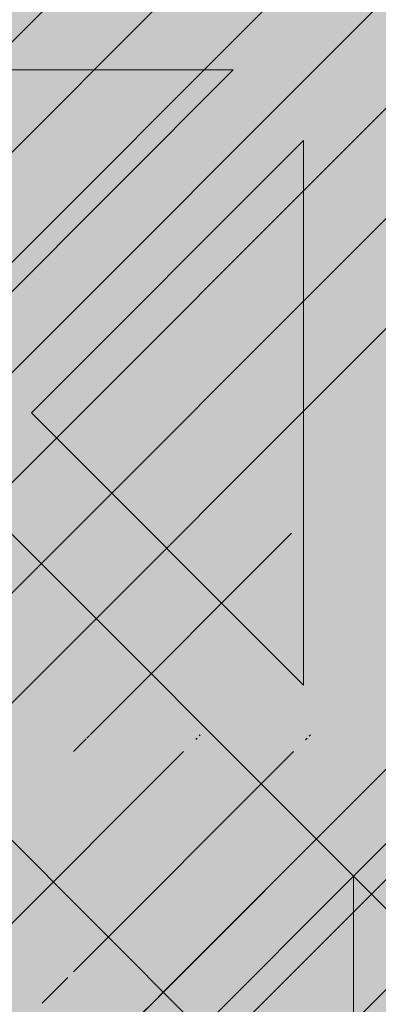
# Model space of a CAD drawing. Units: inches. Extents: x 844 to 2234, y 346 to 1084.
# Tile 11 of 93: x 1122.002 to 1122.921, y 691.183 to 693.702. Entities that reach past the tile are written whole.
import ezdxf

# ---------------------------------------------------------------- set-up
doc = ezdxf.new("R2010")
doc.units = ezdxf.units.IN
doc.header["$MEASUREMENT"] = 0
for name, color, linetype, lineweight in [('A-ANNO-DIMS', 2, 'Continuous', 18), ('furniture', 8, 'Continuous', 18), ('RA-AP-01$0$INT', 35, 'Continuous', 5)]:
    doc.layers.add(name, color=color, linetype=linetype, lineweight=lineweight)
doc.layers.add('RA-AP-01$0$FURN', color=3, linetype='Continuous')
doc.layers.add('RA-AP-01$0$WOOD', color=64, linetype='Continuous')
doc.styles.get("Standard").update_dxf_attribs({"font": 'arial.ttf'})
doc.dimstyles.get("Standard").update_dxf_attribs({"dimtxt": 6, "dimasz": 3, "dimexe": 0.18, "dimexo": 0.0625, "dimgap": 0.09, "dimtad": 0, "dimtih": 1, "dimtoh": 1, "dimdec": 1, "dimzin": 0, "dimdsep": 46, "dimlunit": 3, "dimtxsty": 'Standard', "dimblk": 'ARCHTICK', "dimcen": 0.09, "dimadec": 0, "dimazin": 0, "dimtfac": 1, "dimtdec": 1, "dimtofl": 0, "dimtmove": 0, "dimatfit": 3, "dimfxl": 1, "dimtolj": 1, "dimtzin": 0, "dimarcsym": 0})

# ---------------------------------------------------------------- blocks, each defined once
blk = doc.blocks.new('A$C18D01794')
at = {"layer": 'RA-AP-01$0$INT'}
h = blk.add_hatch(color=256, dxfattribs=at)
h.paths.add_polyline_path([(4.585917135068449, -6.356712009588271), (4.555206456959269, -6.35671200958746), (4.555206456959137, -6.387422687716308), (4.874495778835233, -6.706712009592356), (4.90520645695423, -6.676001331474049)])
h.paths.add_polyline_path([(5.255206456948813, -6.387422687716306), (5.255206456948682, -6.356712009605972), (5.224495778822613, -6.356712009605161), (4.905206456953498, -6.676001331474273), (4.935917135072151, -6.706712009592924)])
h.paths.add_polyline_path([(4.935917135072559, -6.706712009592068), (4.905206456953564, -6.737422687710376), (5.255206456951813, -7.087422687708613), (5.255206456951549, -7.026001331471008)])
h.paths.add_polyline_path([(4.555206456956399, -7.026001331471013), (4.555206456956134, -7.087422687708616), (4.905206456953821, -6.737422687710943), (4.874495778835166, -6.70671200959229)])
h = blk.add_hatch(color=256, dxfattribs=at)
h.paths.add_polyline_path([(4.585917135068448, -6.356712009588273), (4.614201406330596, -6.356712009589021), (4.668846067270487, -6.411356670531338), (4.723490728212344, -6.356712009591912), (4.771774999457151, -6.35671200959319), (4.826419660396886, -6.411356670535356), (4.862780050090322, -6.374996280843536), (4.844495778842715, -6.356712009595112), (4.862780050090411, -6.356712009595595), (4.905206456960182, -6.399138416468211), (4.947632863832445, -6.356712009597838), (4.965917135079675, -6.356712009598322), (4.947632863831759, -6.374996280845421), (4.983993253523576, -6.411356670538857), (5.038637914464627, -6.356712009600247), (5.08692218571208, -6.356712009601523), (5.141566846649976, -6.411356670541852), (5.196211507589851, -6.356712009604411), (5.224495778822615, -6.356712009605161), (4.905206456953975, -6.676001331473793)])
h.paths.add_polyline_path([(4.895206456956031, -6.637717060225675), (4.895206456958921, -6.528427738347902), (4.840561796018589, -6.583072399285802)], flags=16)
h.paths.add_polyline_path([(4.915206456955638, -6.637717060226121), (4.969851117895509, -6.583072399288678), (4.915206456957609, -6.528427738348344)], flags=16)
h.paths.add_polyline_path([(4.826419660395175, -6.568930263661755), (4.881064321335613, -6.514285602723745), (4.771774999456703, -6.514285602720857)], flags=16)
h.paths.add_polyline_path([(4.983993253519558, -6.568930263665262), (5.038637914460456, -6.514285602726792), (4.929348592581548, -6.514285602724816)], flags=16)
h.paths.add_polyline_path([(4.881064321336025, -6.494285602723742), (4.826419660397532, -6.439640941782821), (4.771774999457062, -6.494285602720859)], flags=16)
h.paths.add_polyline_path([(4.929348592582019, -6.494285602724817), (5.038637914460982, -6.494285602726792), (4.983993253522945, -6.439640941786327)], flags=16)
h.paths.add_polyline_path([(4.895206456960191, -6.480143467100443), (4.895206456962115, -6.407422687715913), (4.876922185715016, -6.389138416467584), (4.840561796021581, -6.425498806159401)], flags=16)
h.paths.add_polyline_path([(4.915206456958487, -6.480143467100889), (4.969851117899527, -6.425498806162279), (4.933490728206909, -6.389138416468043), (4.9152064569598, -6.40742268771434)], flags=16)
h.paths.add_polyline_path([(4.757632863832376, -6.480143467096812), (4.812277524772842, -6.425498806158772), (4.757632863834348, -6.370854145217844)], flags=16)
h.paths.add_polyline_path([(4.737632863832376, -6.480143467096286), (4.737632863834348, -6.370854145217375), (4.682988202893906, -6.425498806155385)], flags=16)
h.paths.add_polyline_path([(5.05278005008503, -6.480143467103376), (5.052780050087917, -6.370854145224413), (4.998135389146995, -6.425498806162908)], flags=16)
h.paths.add_polyline_path([(5.072780050085024, -6.480143467103744), (5.127424711025931, -6.42549880616527), (5.072780050087916, -6.370854145224832)], flags=16)
h.paths.add_polyline_path([(4.935917135072783, -6.706712009592292), (5.255206456948811, -6.387422687716309), (5.255206456948932, -6.415706958964177), (5.200561796010279, -6.470351619902839), (5.255206456949403, -6.524996280841948), (5.25520645694961, -6.5732805520894), (5.200561796009787, -6.627925213029239), (5.236922185702417, -6.664285602721864), (5.255206456949919, -6.646001331474357), (5.255206456949998, -6.664285602721898), (5.212780050078687, -6.706712009592262), (5.25520645695036, -6.749138416463932), (5.255206456950438, -6.767422687711313), (5.236922185702424, -6.749138416463297), (5.200561796009796, -6.785498806155928), (5.255206456950753, -6.840143467096874), (5.25520645695096, -6.888427738341682), (5.200561796010322, -6.943072399282328), (5.255206456951428, -6.997717060223427), (5.255206456951547, -7.026001331471006)])
h.paths.add_polyline_path([(5.042988202883395, -6.785498806155427), (5.097632863823085, -6.840143467095101), (5.097632863822622, -6.730854145216193)], flags=16)
h.paths.add_polyline_path([(5.028846067259663, -6.771356670531693), (5.083490728198774, -6.716712009592573), (4.974201406321001, -6.716712009593042)], flags=16)
h.paths.add_polyline_path([(5.117632863823087, -6.840143467095186), (5.172277524762331, -6.785498806155926), (5.11763286382262, -6.730854145216225)], flags=16)
h.paths.add_polyline_path([(5.08349072819877, -6.696712009593886), (5.028846067259652, -6.642067348654775), (4.974201406320998, -6.696712009593438)], flags=16)
h.paths.add_polyline_path([(5.131774999446817, -6.854285602718917), (5.186419660386065, -6.799640941779662), (5.241064321325782, -6.854285602719365)], flags=17)
h.paths.add_polyline_path([(5.131774999446228, -6.716712009592374), (5.186419660386065, -6.771356670532194), (5.222780050079488, -6.734996280838764), (5.204495778832781, -6.716712009592063)], flags=16)
h.paths.add_polyline_path([(5.097632863822613, -6.682569873970264), (5.097632863823061, -6.573280552091354), (5.042988202883383, -6.627925213031044)], flags=16)
h.paths.add_polyline_path([(5.131774999446899, -6.874285602718915), (5.241064321325809, -6.874285602719364), (5.186419660386591, -6.928930263658598)], flags=17)
h.paths.add_polyline_path([(5.131774999446226, -6.696712009594078), (5.204495778830767, -6.696712009594374), (5.22278005007868, -6.67842773834687), (5.186419660386049, -6.642067348654249)], flags=16)
h.paths.add_polyline_path([(5.11763286382262, -6.682569873970225), (5.17227752476232, -6.627925213030515), (5.117632863823064, -6.573280552091267)], flags=16)
h.paths.add_polyline_path([(5.186419660386069, -6.613783077405491), (5.241064321325754, -6.559138416465795), (5.131774999446791, -6.559138416466263)], flags=16)
h.paths.add_polyline_path([(5.131774999446872, -6.539138416466263), (5.24106432132578, -6.539138416465794), (5.186419660386554, -6.484493755526573)], flags=16)
h.paths.add_polyline_path([(5.255206456951811, -7.08742268770861), (5.255206456951895, -7.106712009588038), (4.555206456956052, -7.106712009588038), (4.555206456956136, -7.087422687708617), (4.905206456953973, -6.737422687710788)])
h.paths.add_polyline_path([(4.983993253513404, -6.8444937555241), (4.92934859257295, -6.899138416462108), (5.03863791445186, -6.899138416465014)], flags=16)
h.paths.add_polyline_path([(4.969851117889988, -6.83035161990006), (4.915206456952556, -6.775706958960171), (4.915206456949648, -6.884996280837944)], flags=16)
h.paths.add_polyline_path([(4.929348592572535, -6.919138416462105), (4.983993253511019, -6.973783077403037), (5.038637914451496, -6.919138416465012)], flags=16)
h.paths.add_polyline_path([(5.052780050074912, -6.93328055208906), (4.998135389134438, -6.987925213027088), (5.052780050072919, -7.042569873968025)], flags=16)
h.paths.add_polyline_path([(5.07278005007491, -6.933280552089588), (5.072780050072918, -7.042569873968497), (5.127424711013374, -6.987925213030498)], flags=16)
h.paths.add_polyline_path([(4.89520645695295, -6.775706958959721), (4.840561796013067, -6.830351619897157), (4.895206456950961, -6.884996280837494)], flags=16)
h.paths.add_polyline_path([(4.915206456948365, -6.933280552085403), (4.915206456946434, -7.006001331471951), (4.933490728192729, -7.024285602719066), (4.969851117886972, -6.987925213026453)], flags=16)
h.paths.add_polyline_path([(4.881064321327021, -6.899138416461022), (4.82641966038902, -6.84449375552057), (4.771774999448108, -6.899138416459029)], flags=16)
h.paths.add_polyline_path([(4.895206456950073, -6.933280552084951), (4.840561796009022, -6.987925213023558), (4.876922185700835, -7.024285602716997), (4.895206456948749, -7.006001331469487)], flags=16)
h.paths.add_polyline_path([(4.983993253510392, -7.0020673486505), (4.947632863816944, -7.038427738342319), (4.965917135064043, -7.05671200959023), (5.038637914448995, -7.056712009591555)], flags=16)
h.paths.add_polyline_path([(4.881064321326543, -6.91913841646102), (4.771774999447578, -6.919138416459031), (4.826419660385607, -6.973783077399508)], flags=16)
h.paths.add_polyline_path([(4.905206456946447, -7.014285602717636), (4.862780050074785, -7.056712009588352), (4.947632863816685, -7.056712009589775)], flags=16)
h.paths.add_polyline_path([(5.14156684663679, -7.002067348654549), (5.086922185696452, -7.056712009592438), (5.196211507574223, -7.056712009594425)], flags=16)
h.paths.add_polyline_path([(4.8264196603837, -7.002067348646972), (4.771774999442643, -7.056712009585575), (4.8444957788276, -7.056712009587508), (4.862780050075511, -7.038427738340416)], flags=16)
h.paths.add_polyline_path([(4.812277524760289, -6.98792521302292), (4.757632863822258, -6.933280552082447), (4.757632863819352, -7.042569873961408)], flags=16)
h.paths.add_polyline_path([(4.73763286382226, -6.933280552082079), (4.682988202881349, -6.987925213020536), (4.737632863819352, -7.04256987396099)], flags=16)
h.paths.add_polyline_path([(4.723490728195188, -7.056712009584289), (4.668846067257299, -7.002067348643949), (4.614201406317417, -7.056712009581383)], flags=16)
h.paths.add_polyline_path([(4.597632863829262, -6.706712009592262), (4.555206456957951, -6.664285602721896), (4.555206456958029, -6.646001331474357), (4.573490728205535, -6.664285602721864), (4.609851117898167, -6.627925213029238), (4.555206456958338, -6.573280552089402), (4.555206456958546, -6.524996280841952), (4.60985111789767, -6.470351619902839), (4.555206456959015, -6.415706958964177), (4.555206456959138, -6.387422687716309), (4.874495778835167, -6.70671200959229), (4.5552064569564, -7.026001331471015), (4.555206456956523, -6.997717060223433), (4.609851117897629, -6.94307239928233), (4.555206456956988, -6.888427738341681), (4.555206456957198, -6.840143467096881), (4.609851117898153, -6.78549880615593), (4.573490728205528, -6.749138416463297), (4.555206456957507, -6.76742268771132), (4.555206456957585, -6.749138416463933)])
h.paths.add_polyline_path([(4.712780050085332, -6.730854145216195), (4.712780050084863, -6.840143467095105), (4.767424711024555, -6.785498806155427)], flags=16)
h.paths.add_polyline_path([(4.726922185709173, -6.716712009592573), (4.781566846648288, -6.771356670531693), (4.836211507586949, -6.716712009593043)], flags=16)
h.paths.add_polyline_path([(4.692780050085327, -6.730854145216225), (4.638135389145619, -6.785498806155928), (4.692780050084865, -6.840143467095185)], flags=16)
h.paths.add_polyline_path([(4.726922185709182, -6.696712009593886), (4.836211507586949, -6.696712009593436), (4.7815668466483, -6.642067348654773)], flags=16)
h.paths.add_polyline_path([(4.678637914461726, -6.71671200959237), (4.605917135075169, -6.716712009592063), (4.587632863828464, -6.734996280838766), (4.623993253521887, -6.771356670532195)], flags=16)
h.paths.add_polyline_path([(4.712780050085336, -6.68256987397026), (4.767424711024568, -6.627925213031042), (4.71278005008489, -6.573280552091352)], flags=16)
h.paths.add_polyline_path([(4.678637914461726, -6.696712009594076), (4.623993253521899, -6.642067348654247), (4.587632863829271, -6.67842773834687), (4.605917135077185, -6.696712009594376)], flags=16)
h.paths.add_polyline_path([(4.692780050085336, -6.682569873970228), (4.692780050084889, -6.573280552091267), (4.638135389145632, -6.627925213030515)], flags=16)
h.paths.add_polyline_path([(4.623993253521885, -6.799640941779662), (4.678637914461131, -6.854285602718915), (4.56934859258217, -6.854285602719365)], flags=17)
h.paths.add_polyline_path([(4.623993253521901, -6.613783077405509), (4.678637914461158, -6.559138416466263), (4.569348592582195, -6.559138416465795)], flags=16)
h.paths.add_polyline_path([(4.678637914461051, -6.874285602718915), (4.623993253521361, -6.928930263658598), (4.569348592582143, -6.874285602719364)], flags=17)
h.paths.add_polyline_path([(4.678637914461076, -6.539138416466263), (4.623993253521399, -6.484493755526573), (4.569348592582167, -6.539138416465796)], flags=16)
h = blk.add_hatch(color=256, dxfattribs=at)
h.paths.add_polyline_path([(4.905206456953579, -6.70671200959253), (4.905206456953751, -6.676001331474523), (4.874495778835229, -6.706712009592358)])
h.paths.add_polyline_path([(4.935917135071924, -6.706712009592703), (4.905206456953583, -6.706712009592529), (4.90520645695341, -6.737422687710532)])
h = blk.add_hatch(color=256, dxfattribs=at)
h.paths.add_polyline_path([(4.905206456953409, -6.737422687710532), (4.90520645695358, -6.706712009592529), (4.874495778835235, -6.706712009592359)])
h.paths.add_polyline_path([(4.935917135071928, -6.706712009592703), (4.905206456953754, -6.676001331474527), (4.905206456953582, -6.706712009592529)])
h = blk.add_hatch(color=256, dxfattribs=at)
h.paths.add_polyline_path([(4.895206456952951, -6.77570695895972), (4.840561796013068, -6.830351619897156), (4.895206456950958, -6.884996280837495)])
h.paths.add_polyline_path([(4.915206456949649, -6.884996280837942), (4.969851117889987, -6.830351619900054), (4.915206456952556, -6.775706958960171)])
h.paths.add_polyline_path([(5.038637914451862, -6.899138416465013), (4.983993253513403, -6.8444937555241), (4.929348592572953, -6.899138416462106)])
h.paths.add_polyline_path([(4.929348592572535, -6.919138416462105), (4.983993253511018, -6.973783077403037), (5.038637914451497, -6.919138416465012)])
h.paths.add_polyline_path([(4.915206456948366, -6.933280552085397), (4.915206456946433, -7.006001331471951), (4.93349072819273, -7.024285602719068), (4.969851117886972, -6.987925213026454)])
h.paths.add_polyline_path([(5.038637914448995, -7.056712009591553), (4.983993253510389, -7.002067348650502), (4.947632863816946, -7.038427738342318), (4.965917135064043, -7.05671200959023)])
h.paths.add_polyline_path([(5.05278005007292, -7.042569873968023), (5.05278005007491, -6.933280552089059), (4.998135389134438, -6.987925213027088)])
h.paths.add_polyline_path([(5.07278005007292, -7.042569873968496), (5.127424711013374, -6.987925213030498), (5.072780050074909, -6.933280552089588)])
h.paths.add_polyline_path([(5.141566846636789, -7.002067348654547), (5.086922185696449, -7.056712009592438), (5.196211507574223, -7.056712009594425)])
h.paths.add_polyline_path([(4.947632863816688, -7.056712009589774), (4.905206456946449, -7.014285602717634), (4.862780050074784, -7.056712009588353)])
h.paths.add_polyline_path([(4.840561796009025, -6.987925213023556), (4.876922185700834, -7.024285602716997), (4.895206456948747, -7.006001331469488), (4.895206456950075, -6.933280552084953)])
h.paths.add_polyline_path([(4.88106432132654, -6.919138416461021), (4.771774999447577, -6.919138416459031), (4.826419660385606, -6.973783077399508)])
h.paths.add_polyline_path([(4.881064321327019, -6.899138416461022), (4.826419660389019, -6.844493755520571), (4.771774999448108, -6.89913841645903)])
h.paths.add_polyline_path([(4.757632863819352, -7.042569873961409), (4.812277524760284, -6.987925213022922), (4.757632863822259, -6.933280552082447)])
h.paths.add_polyline_path([(4.8264196603837, -7.002067348646974), (4.771774999442646, -7.056712009585575), (4.844495778827599, -7.05671200958751), (4.862780050075512, -7.038427738340417)])
h.paths.add_polyline_path([(4.737632863819352, -7.042569873960988), (4.737632863822258, -6.933280552082078), (4.682988202881349, -6.987925213020538)])
h.paths.add_polyline_path([(4.668846067257299, -7.002067348643952), (4.61420140631742, -7.056712009581384), (4.723490728195189, -7.056712009584292)])
for p, q in [((4.905206456953753, -6.676001331474525), (4.905206456953409, -6.737422687710532)), ((4.874495778835167, -6.70671200959229), (4.555206456956399, -7.026001331471013)), ((4.874495778835233, -6.706712009592356), (4.905206456953409, -6.737422687710532)), ((4.935917135071927, -6.706712009592701), (4.905206456953407, -6.737422687710532)), ((4.905206456953975, -6.737422687710788), (4.555206456956136, -7.087422687708617)), ((4.905206456953975, -6.737422687710788), (5.255206456951811, -7.087422687708611)), ((4.89520645695295, -6.775706958959723), (4.840561796013068, -6.830351619897156)), ((4.895206456950959, -6.884996280837494), (4.89520645695295, -6.775706958959723)), ((4.895206456950956, -6.884996280837492), (4.840561796013068, -6.830351619897156)), ((4.881064321327019, -6.899138416461022), (4.82641966038902, -6.844493755520572)), ((4.771774999448109, -6.899138416459031), (4.881064321327019, -6.899138416461022))]:
    blk.add_line(p, q, dxfattribs=at)
blk = doc.blocks.new('A$C32926AE1')
at = {"layer": 'RA-AP-01$0$FURN'}
h = blk.add_hatch(dxfattribs=at)
h.set_pattern_fill('ANSI31', color=256, scale=0.1, style=0)
h.set_pattern_definition([(45, (0, 0), (-0.0088388347648318, 0.0088388347648318), [])])
edge = h.paths.add_edge_path(flags=16)
edge.add_arc((4.904771284329206, 4.246793130718756), 0.2603971832811541, 75.22398030683196, 104.7760196931204)
edge.add_arc((4.904771284329206, 4.246793130718756), 0.2603971832811541, 75.223980306832, 104.77601969312039, ccw=False)
edge = h.paths.add_edge_path(flags=16)
edge.add_arc((4.904771284329206, 4.067062675376612), 0.2603971832811541, 255.2239803068796, 284.776019693168)
edge.add_arc((4.904771284329206, 4.067062675376612), 0.2603971832811541, 255.22398030687958, 284.77601969316805, ccw=False)
edge = h.paths.add_edge_path(flags=0)
edge.add_arc((4.904771284329206, 4.067062675376612), 0.2603971832811541, 255.2239803068796, 284.776019693168)
edge.add_arc((4.904771284329206, 4.067062675376612), 0.2603971832811541, 255.22398030687958, 284.77601969316805, ccw=False)
edge = h.paths.add_edge_path(flags=0)
edge.add_arc((4.904771284329206, 4.067062675376612), 0.2603971832811541, 255.2239803068796, 284.776019693168)
edge.add_arc((4.904771284329206, 4.067062675376612), 0.2603971832811541, 255.22398030687958, 284.77601969316805, ccw=False)
edge = h.paths.add_edge_path()
edge.add_arc((4.604388392048174, 4.588829985554312), 0.1599999999999918, 342.3781640246255, 354.4317409793762)
edge.add_arc((5.090145208887507, 4.43216705527679), 0.3503971832811637, 162.0091218307731, 180.3186872093483)
edge.add_arc((5.205154176610243, 4.588829985554953), 0.1599999999999917, 185.5682590208461, 197.6218359767349)
edge.add_arc((4.904771284329229, 4.246793130718735), 0.3503971832811761, 72.00912183053516, 107.9908781690354)
edge.add_arc((9.535952835716557, 4.28682295566602), 4.798342501046485, 178.2875002453811, 181.5576802719453)
edge.add_arc((4.719397359771122, 4.43216705527679), 0.3503971832811637, 359.6813127906516, 377.9908781692269)
edge.add_arc((9.535967292294904, 4.286822350292874), 4.778371420254705, 178.2965938931842, 181.5667745797229)
edge.add_arc((4.719397359771122, 4.43216705527679), 0.3303971832811637, 359.6813127906516, 377.9908781692269)
edge.add_arc((0.2735752763637294, 4.286822350292874), 4.7783714202547, 358.4332254202771, 361.7034061068158)
edge.add_arc((5.061434214606998, 4.732549947558029), 0.1600000000000254, 252.3781640250584, 264.4317409792362)
edge.add_arc((4.748108354051257, 4.732549947558012), 0.1600000000000541, 275.5682590208426, 287.6218359759532)
edge.add_arc((4.604388392048115, 4.588829985554317), 0.1800000000000505, 342.3567572500182, 349.3735009646207)
edge.add_arc((5.205154176610254, 4.588829985554976), 0.1800000000000069, 190.6264990356027, 197.6432427513933)
edge.add_arc((5.061434214607106, 4.732549947558013), 0.1800000000000424, 252.3567572496606, 259.3735009644582)
edge.add_arc((4.904771284329208, 4.246793130718737), 0.3303971832811676, 71.99844483668534, 108.0015551637021)
edge.add_arc((4.748108354051414, 4.732549947558045), 0.1800000000000547, 280.6264990355479, 287.6432427495938)
edge.add_arc((5.090145208887514, 4.432167055276789), 0.2803971832811691, 162.8706300666893, 180.816523289902)
edge.add_arc((4.719397359771136, 4.432167055276689), 0.2803971832811534, 359.183476710103, 377.1293699333214)
edge.add_arc((4.904771284329222, 4.246793130718737), 0.2803971832811769, 72.87063006672916, 107.1293699332334)
edge.add_arc((5.090145208887522, 4.432167055276788), 0.2603971832811776, 165.2239803068007, 180.9953123810312)
edge.add_arc((4.719397359771141, 4.432167055276699), 0.2603971832811458, 359.0046876189768, 374.7760196932087)
edge.add_arc((5.090145208887507, 4.43216705527679), 0.3303971832811637, 162.0091218307731, 180.3186872093483)
edge.add_arc((9.53595427642584, 4.285015535491528), 4.728345371032053, 178.265043920078, 181.5679956281801)
edge.add_arc((0.2735882922327999, 4.285015535491582), 4.728345371032045, 358.4320043718193, 361.7349560799204)
edge.add_arc((9.535953591267507, 4.284458026472751), 4.708343996644348, 178.2573054306777, 181.5704995759608)
edge.add_arc((0.273588977391114, 4.284458026472785), 4.708343996644358, 358.4295004240388, 361.7426945693213)
edge.add_arc((0.2735889773911131, 4.029397779622582), 4.708343996644359, 358.2573054306787, 361.5704995759613)
edge.add_arc((9.535953591267518, 4.029397779622618), 4.708343996644359, 178.4295004240391, 181.7426945693223)
edge.add_arc((0.2735882922327901, 4.028840270603786), 4.728345371032054, 358.2650439200796, 361.5679956281808)
edge.add_arc((9.53595427642584, 4.028840270603841), 4.728345371032054, 178.4320043718199, 181.7349560799219)
edge.add_arc((0.2735752763637302, 4.027033455802493), 4.778371420254699, 358.2965938931842, 361.5667745797229)
edge.add_arc((4.719397359771122, 3.881688750818578), 0.3303971832811637, 342.0091218307731, 360.3186872093484)
edge.add_arc((5.090145208887507, 3.881688750818578), 0.3303971832811637, 179.6813127906516, 197.9908781692269)
edge.add_arc((9.535967292294904, 4.027033455802493), 4.778371420254705, 178.433225420277, 181.7034061068158)
edge.add_arc((4.719397359771122, 3.881688750818578), 0.3503971832811637, 342.0091218307731, 360.3186872093484)
edge.add_arc((9.53595283571655, 4.027032850429349), 4.79834250104648, 178.4423197280546, 181.7124997546188)
edge.add_arc((4.719397359771141, 3.881688750818669), 0.2603971832811458, 345.2239803067913, 360.9953123810232)
edge.add_arc((5.090145208887522, 3.88168875081858), 0.2603971832811776, 179.0046876189687, 194.7760196931993)
edge.add_arc((4.904771284329222, 4.067062675376631), 0.2803971832811769, 252.8706300667665, 287.1293699332708)
edge.add_arc((4.719397359771136, 3.881688750818678), 0.2803971832811534, 342.8706300666787, 360.8165232898969)
edge.add_arc((5.090145208887514, 3.881688750818579), 0.2803971832811691, 179.183476710098, 197.1293699333106)
edge.add_arc((4.748108354051414, 3.581305858537323), 0.1800000000000547, 72.3567572504062, 79.37350096445199)
edge.add_arc((4.904771284329208, 4.067062675376631), 0.3303971832811676, 251.9984448362979, 288.0015551633146)
edge.add_arc((5.061434214607106, 3.581305858537355), 0.1800000000000424, 100.6264990355418, 107.6432427503394)
edge.add_arc((5.205154176610254, 3.725025820540392), 0.1800000000000069, 162.3567572486066, 169.3735009643972)
edge.add_arc((4.604388392048115, 3.725025820541051), 0.1800000000000505, 10.62649903537925, 17.64324274998182)
edge.add_arc((4.748108354051257, 3.581305858537356), 0.1600000000000541, 72.37816402404681, 84.43174097915735)
edge.add_arc((4.904771284329229, 4.067062675376632), 0.3503971832811761, 252.0091218309645, 287.9908781694648)
edge.add_arc((5.061434214606998, 3.581305858537339), 0.1600000000000254, 95.56825902076373, 107.6218359749416)
edge.add_arc((5.205154176610243, 3.725025820540414), 0.1599999999999917, 162.3781640232651, 174.4317409791539)
edge.add_arc((5.090145208887507, 3.881688750818578), 0.3503971832811637, 179.6813127906516, 197.9908781692269)
edge.add_arc((4.604388392048174, 3.725025820541056), 0.1599999999999918, 5.568259020623824, 17.62183597537444)
edge.add_arc((0.2735897329420762, 4.28682295566602), 4.798342501046482, 358.4423197280547, 361.7124997546188)
edge.add_arc((0.2735897329420691, 4.027032850429348), 4.798342501046489, 358.2875002453812, 361.5576802719453)
at = {"layer": 'RA-AP-01$0$WOOD'}
h = blk.add_hatch(color=256, dxfattribs=at)
h.dxf.hatch_style = 1
h.paths.add_polyline_path([(5.157430609644524, 4.573483066760929, -0.1009492694046607), (5.155401577623758, 4.593365984175333, -0.1842662638101597), (5.172249623284174, 4.638795604568598, 0.2056608120311276), (5.179560981299304, 4.661316324430096, 0.3614336704623542), (5.134352340494423, 4.706524965234944, 0.2056608120311297), (5.111831620632933, 4.699213607219793, -0.1842662638101113), (5.066402000239693, 4.682365561559342, -0.1055311479399994), (5.045656153913092, 4.68467289944697, 0.1567636581983829), (4.763886414745334, 4.684672899446966, -0.1055311479399895), (4.743140568418733, 4.68236556155934, -0.1842662638100833), (4.6977109480255, 4.69921360721979, 0.2056608120302612), (4.675190228164109, 4.706524965234949, 0.3614336704708441), (4.629981587358889, 4.66131632442871, 0.2056608120245944), (4.637292945374126, 4.638795604567974, -0.1842662638101024), (4.654140991034615, 4.59336598417475, -0.1009492694055169), (4.652111959013835, 4.573483066760181, 0.021410119221476), (4.629748025606143, 4.156712009541676, 0.0214101192214795), (4.652111959013809, 3.739940952323101, -0.1009492694059586), (4.654140991034615, 3.720058034908448, -0.1842662638100975), (4.637292945374126, 3.674628414515226, 0.2056608120245705), (4.629981587358889, 3.652107694654492, 0.3614336704708879), (4.675190228164113, 3.606899053848249, 0.2056608120302384), (4.697710948025501, 3.614210411863408, -0.1842662638100995), (4.743140568418738, 3.63105845752386, -0.1055311479402541), (4.763886414745388, 3.628751119636215, 0.1567636581983776), (5.045656153913137, 3.628751119636244, -0.1055311479397538), (5.066402000239692, 3.631058457523857, -0.1842662638101067), (5.111831620632931, 3.614210411863407, 0.2056608120310924), (5.134352340494417, 3.606899053848256, 0.3614336704624001), (5.179560981299307, 3.652107694653103, 0.2056608120311314), (5.172249623284175, 3.6746284145146, -0.1842662638101402), (5.155401577623758, 3.72005803490786, -0.1009492694051366), (5.15743060964455, 3.739940952322354, 0.0214101192215073), (5.179794543052287, 4.156712009541468, 0.0214101192215252)])
h.paths.add_polyline_path([(4.639748609479751, 4.156712009541513, 0.0213537860821624), (4.661970494867118, 3.741887061152232, -0.094075836301374), (4.664143710413708, 3.7196126951003, -0.1824818158568985), (4.644813765429836, 3.668037719127816, 0.2056608120245319), (4.639939526753007, 3.653023905887301, 0.3614336704710246), (4.676106439397173, 3.616856993242342, 0.2056608120302234), (4.691120252638095, 3.621731231919122, -0.1824818158602558), (4.742695228611606, 3.641061176902986, -0.1029891339458722), (4.766991894714349, 3.638256818950944, 0.156709409989566), (5.042550673941472, 3.638256818950105, -0.102989133958497), (5.066847340047078, 3.641061176902949, -0.1824818158594995), (5.118422316020358, 3.621731231919103, 0.2056608120311416), (5.133436129261316, 3.616856993242346, 0.3614336704621468), (5.169603041905217, 3.653023905886178, 0.2056608120310986), (5.164728803228477, 3.668037719127177, -0.1824818158565612), (5.145398858244737, 3.719612695099578, -0.0940758363009313), (5.147572073791232, 3.741887061151398, 0.0213537860822023), (5.169793959178681, 4.156712009541451, 0.0213537860822226), (5.147572073791203, 4.571536957931898, -0.0940758363005034), (5.145398858244737, 4.59381132398362, -0.1824818158565587), (5.164728803228476, 4.645386299956021, 0.2056608120311045), (5.169603041905216, 4.66040011319702, 0.3614336704621845), (5.133436129261313, 4.696567025840856, 0.2056608120310773), (5.118422316020359, 4.691692787164098, -0.182481815859508), (5.066847340047078, 4.67236284218025, -0.1029891339584606), (5.04255067394148, 4.675167200133092, 0.156709409989566), (4.766991894714357, 4.675167200132257, -0.1029891339458842), (4.742695228611611, 4.672362842180213, -0.1824818158602725), (4.691120252638095, 4.691692787164077, 0.2056608120302152), (4.676106439397174, 4.696567025840858, 0.3614336704710363), (4.639939526753005, 4.660400113195899, 0.2056608120245495), (4.644813765429837, 4.645386299955384, -0.1824818158568934), (4.664143710413708, 4.593811323982902, -0.0940758363009187), (4.661970494867149, 4.571536957931074, 0.021353786082177)], flags=16)
h.paths.add_polyline_path([(5.129794543052235, 4.432167055276933, -0.0141661062790638), (5.130152669293814, 4.156927903047693, -0.0141661062790647), (5.129794543052234, 3.881688750818433, -0.0785247771143638), (5.10979738006795, 3.755143611847103, 0.0945969212073497), (5.105408519571111, 3.717898134952927, 0.1043170707844957), (5.116074640131521, 3.670385395016088, 0.1043170707864965), (5.068561900193738, 3.681051515576561, 0.09459692119553), (5.031316423304057, 3.676662655080835, -0.1580239521427272), (4.778226145355827, 3.676662655080367, 0.0945969211986668), (4.740980668464973, 3.681051515576592, 0.1043170707882822), (4.693467928526415, 3.670385395015844, 0.1043170707867916), (4.704134049087309, 3.717898134953662, 0.0945969211972894), (4.69974518859162, 3.755143611844042, -0.0785247771163196), (4.679748025606343, 3.881688750818406, -0.0141661062790663), (4.679389899364763, 4.156927903047693, -0.0141661062790672), (4.679748025606343, 4.432167055276998, -0.0785247771163064), (4.699745188591625, 4.55871219425134, 0.094596921197333), (4.704134049087308, 4.595957671141738, 0.1043170707867205), (4.693467928526416, 4.643470411079523, 0.1043170707882628), (4.740980668464965, 4.632804290518776, 0.0945969211988114), (4.778226145355874, 4.637193151015016, -0.158023952142669), (5.031316423304015, 4.637193151014546, 0.0945969211956361), (5.068561900193736, 4.632804290518806, 0.1043170707864979), (5.11607464013152, 4.643470411079278, 0.1043170707844617), (5.105408519571112, 4.595957671142455, 0.0945969212074597), (5.109797380067959, 4.558712194248236, -0.0785247771143467)], flags=0)
h.paths.add_polyline_path([(5.119794532311105, 4.432259799204851, -0.0142000800617244), (5.120156169157484, 4.156927903047701, -0.0142000800617277), (5.119794532311105, 3.881596006890482, -0.0784894509520253), (5.100273383573699, 3.758192358677797, 0.0940138827242913), (5.095413455884425, 3.717477693979438, 0.0606271852308753), (5.099615656341024, 3.686844378806616, 0.0606271852322524), (5.068982341167493, 3.691046579263239, 0.0940138827010453), (5.028267676478798, 3.686186651576848, -0.1580706864508061), (4.781274892180912, 3.686186651576435, 0.0940138827026903), (4.740560227491556, 3.691046579263279, 0.0606271852339895), (4.709926912317155, 3.686844378806508, 0.0606271852329405), (4.714129112773991, 3.717477693980356, 0.094013882701304), (4.709269185087677, 3.758192358669163, -0.0784894509577193), (4.689748036347473, 3.881596006890469, -0.014200080061729), (4.689386399501094, 4.156927903047709, -0.0142000800617217), (4.689748036347473, 4.432259799204808, -0.078489450957724), (4.709269185087651, 4.555663447426125, 0.0940138827014585), (4.714129112773992, 4.596378112114996, 0.0606271852329731), (4.709926912317154, 4.62701142728886, 0.0606271852340196), (4.74056022749157, 4.622809226832087, 0.0940138827024997), (4.781274892180847, 4.627669154518912, -0.1580706864508359), (5.028267676478777, 4.627669154518526, 0.0940138827010946), (5.068982341167492, 4.622809226832129, 0.060627185232254), (5.099615656341024, 4.627011427288751, 0.0606271852308727), (5.095413455884425, 4.59637811211593, 0.0940138827241088), (5.100273383573675, 4.555663447417647, -0.0784894509520978)], flags=0)
h.paths.add_polyline_path([(5.06978912287499, 4.430218106756144, -0.014241683694547), (5.070173729147532, 4.156927903047672, -0.0142416836945458), (5.06978912287499, 3.883637699339223, -0.0800609523125196), (5.052662118612511, 3.773463122773442, 0.0526421978001116), (5.04590916754064, 3.740550867606997, 0.0526421977992423), (5.012996912374707, 3.73379791653534, -0.1583028414718258), (4.796545656286308, 3.73379791653451, 0.0526421978034211), (4.763633401117837, 3.740550867607021, 0.0526421978018622), (4.756880450045755, 3.773463122774558, -0.0800609523117106), (4.739753445783639, 3.883637699339268, -0.0142416836945435), (4.739368839511098, 4.156927903047671, -0.0142416836945477), (4.739753445783639, 4.430218106756155, -0.0800609523116345), (4.75688045004574, 4.540392683320762, 0.052642197801941), (4.763633401117837, 4.573304938488346, 0.0526421978035071), (4.796545656286361, 4.580057889560873, -0.1583028414717561), (5.012996912374669, 4.580057889560039, 0.0526421977993048), (5.04590916754064, 4.57330493848837, 0.0526421978002057), (5.052662118612529, 4.540392683321868, -0.080060952312477)], flags=0)
h.paths.add_polyline_path([(5.049789715110557, 4.43038092723357, -0.0143097550741839), (5.05018085590259, 4.156927903047715, -0.0143097550741854), (5.049789715110558, 3.883474878861827, -0.0800685599149176), (5.03362098255317, 3.779581877367999, 0.0306258898956367), (5.028241146483733, 3.758218888663947, 0.0306258898977031), (5.006878157778253, 3.75283905259408, -0.1583983521624096), (4.802664410878162, 3.752839052594731, 0.0306258898946014), (4.781301422174808, 3.758218888663924, 0.0306258898967912), (4.775921586105202, 3.779581877368794, -0.080068559914251), (4.759752853548071, 3.883474878861786, -0.0143097550741854), (4.759361712756037, 4.156927903047671, -0.0143097550741854), (4.759752853548071, 4.430380927233557, -0.0800685599142479), (4.775921586105193, 4.534273928726546, 0.0306258898968306), (4.781301422174808, 4.555636917431444, 0.0306258898945754), (4.802664410878143, 4.561016753500631, -0.1583983521624168), (5.006878157778244, 4.561016753501291, 0.0306258898977177), (5.028241146483733, 4.555636917431421, 0.0306258898958182), (5.03362098255321, 4.534273928727244, -0.080068559914796)], flags=0)
h.paths.add_polyline_path([(4.999766070382627, 4.428171244713864, -0.0143443147609634), (5.000198441819402, 4.156927903047689, -0.0143443147609612), (4.999766070382627, 3.885684561381556, -0.0784641635803329), (4.987356730658798, 3.799103304488872, -0.1506053783831347), (4.822185837999821, 3.79910330448882, -0.0784641635803318), (4.809776498276007, 3.885684561381509, -0.014344314760963), (4.809344126839227, 4.156927903047677, -0.0143443147609645), (4.809776498276007, 4.428171244713873, -0.0784641635803192), (4.822185837999822, 4.514752501606549, -0.1506053783831338), (4.987356730658798, 4.514752501606494, -0.078464163580285)], flags=0)
h.paths.add_polyline_path([(4.979755254238824, 4.42764379880488, -0.0143772539198268), (4.980205517789977, 4.156927903047693, -0.0143772539198275), (4.979755254238824, 3.886212007290489, -0.0689242507424422), (4.971183264704897, 3.815276770442801, -0.1296645318904179), (4.838359303953726, 3.815276770442746, -0.0689242507424186), (4.829787314419809, 3.886212007290419, -0.0143772539198292), (4.829337050868653, 4.156927903047653, -0.0143772539198325), (4.829787314419809, 4.427643798804946, -0.0689242507424211), (4.838359303953725, 4.498579035652621, -0.1296645318904187), (4.971183264704897, 4.498579035652565, -0.0689242507424401)], flags=0)
h = blk.add_hatch(color=256, dxfattribs=at)
h.dxf.hatch_style = 1
h.paths.add_polyline_path([(5.145398858244737, 4.59381132398362, -0.1824818158565616), (5.164728803228476, 4.645386299956021, 0.2056608120311045), (5.169603041905216, 4.66040011319702, 0.3614336704621845), (5.133436129261313, 4.696567025840856, 0.2056608120310773), (5.118422316020359, 4.691692787164098, -0.182481815859508), (5.066847340047078, 4.67236284218025, -0.1029891339584606), (5.04255067394148, 4.675167200133092, 0.156709409989566), (4.766991894714357, 4.675167200132257, -0.1029891339458842), (4.742695228611611, 4.672362842180213, -0.1824818158602725), (4.691120252638095, 4.691692787164077, 0.2056608120302152), (4.676106439397174, 4.696567025840858, 0.3614336704710363), (4.639939526753005, 4.660400113195899, 0.2056608120245495), (4.644813765429837, 4.645386299955384, -0.1824818158568934), (4.664143710413708, 4.593811323982902, -0.0940758363009187), (4.661970494867149, 4.571536957931074, 0.0213537860821772), (4.639748609479751, 4.156712009541507, 0.0213537860821625), (4.661970494867119, 3.741887061152226, -0.0940758363013071), (4.664143710413708, 3.719612695100309, -0.1824818158569294), (4.644813765429836, 3.668037719127816, 0.2056608120245319), (4.639939526753007, 3.653023905887301, 0.3614336704710246), (4.676106439397173, 3.616856993242342, 0.2056608120302234), (4.691120252638095, 3.621731231919122, -0.1824818158602558), (4.742695228611606, 3.641061176902986, -0.1029891339458722), (4.766991894714349, 3.638256818950944, 0.156709409989566), (5.042550673941472, 3.638256818950105, -0.102989133958497), (5.066847340047078, 3.641061176902949, -0.1824818158594995), (5.118422316020358, 3.621731231919103, 0.2056608120311416), (5.133436129261316, 3.616856993242346, 0.3614336704621468), (5.169603041905217, 3.653023905886178, 0.2056608120310986), (5.164728803228477, 3.668037719127177, -0.1824818158565612), (5.145398858244737, 3.719612695099578, -0.0940758363009313), (5.147572073791232, 3.741887061151398, 0.0213537860822023), (5.169793959178681, 4.156712009541451, 0.0213537860822226), (5.147572073791203, 4.571536957931898, -0.0940758363004996)])
h.paths.add_polyline_path([(5.109797380067958, 4.55871219424824, -0.0785247771143472), (5.129794543052234, 4.432167055276936, -0.0141661062790644), (5.130152669293814, 4.156927903047685, -0.014166106279066), (5.129794543052234, 3.881688750818401, -0.0785247771143517), (5.109797380067946, 3.755143611847092, 0.0945969212073132), (5.105408519571111, 3.717898134952929, 0.1043170707844995), (5.116074640131521, 3.670385395016088, 0.1043170707864965), (5.068561900193738, 3.681051515576561, 0.09459692119553), (5.031316423304057, 3.676662655080835, -0.1580239521427272), (4.778226145355827, 3.676662655080367, 0.0945969211986668), (4.740980668464973, 3.681051515576592, 0.1043170707882822), (4.693467928526415, 3.670385395015844, 0.1043170707867916), (4.704134049087309, 3.717898134953662, 0.0945969211972894), (4.69974518859162, 3.755143611844042, -0.0785247771163196), (4.679748025606343, 3.881688750818406, -0.0141661062790663), (4.679389899364763, 4.156927903047693, -0.0141661062790672), (4.679748025606343, 4.432167055276998, -0.0785247771163064), (4.699745188591625, 4.55871219425134, 0.094596921197333), (4.704134049087308, 4.595957671141738, 0.1043170707867205), (4.693467928526416, 4.643470411079523, 0.1043170707882628), (4.740980668464965, 4.632804290518776, 0.0945969211988114), (4.778226145355874, 4.637193151015016, -0.158023952142669), (5.031316423304015, 4.637193151014546, 0.0945969211956361), (5.068561900193736, 4.632804290518806, 0.1043170707864979), (5.11607464013152, 4.643470411079278, 0.1043170707844617), (5.105408519571112, 4.595957671142455, 0.0945969212074504)], flags=16)
h.paths.add_polyline_path([(5.100273383573655, 4.55566344741771, -0.0784894509521388), (5.119794532311105, 4.432259799204852, -0.0142000800617252), (5.120156169157484, 4.156927903047686, -0.014200080061726), (5.119794532311105, 3.881596006890502, -0.0784894509520446), (5.100273383573696, 3.758192358677786, 0.0940138827242721), (5.095413455884425, 3.717477693979436, 0.0606271852308692), (5.099615656341024, 3.686844378806616, 0.0606271852322522), (5.068982341167493, 3.691046579263239, 0.0940138827010453), (5.028267676478798, 3.686186651576848, -0.1580706864508061), (4.781274892180912, 3.686186651576435, 0.0940138827026903), (4.740560227491556, 3.691046579263279, 0.0606271852339895), (4.709926912317155, 3.686844378806508, 0.0606271852329405), (4.714129112773991, 3.717477693980356, 0.094013882701304), (4.709269185087677, 3.758192358669163, -0.0784894509577193), (4.689748036347473, 3.881596006890469, -0.014200080061729), (4.689386399501094, 4.156927903047709, -0.0142000800617217), (4.689748036347473, 4.432259799204808, -0.078489450957724), (4.709269185087651, 4.555663447426125, 0.0940138827014585), (4.714129112773992, 4.596378112114996, 0.0606271852329731), (4.709926912317154, 4.62701142728886, 0.0606271852340196), (4.74056022749157, 4.622809226832087, 0.0940138827024997), (4.781274892180847, 4.627669154518912, -0.1580706864508359), (5.028267676478777, 4.627669154518526, 0.0940138827010946), (5.068982341167492, 4.622809226832129, 0.060627185232254), (5.099615656341024, 4.627011427288751, 0.0606271852308727), (5.095413455884425, 4.59637811211593, 0.094013882723957)], flags=0)
h.paths.add_polyline_path([(5.04590916754064, 4.57330493848837, 0.0526421978002057), (5.052662118612529, 4.540392683321868, -0.0800609523124783), (5.06978912287499, 4.430218106756142, -0.0142416836945469), (5.070173729147532, 4.156927903047672, -0.0142416836945458), (5.06978912287499, 3.883637699339223, -0.0800609523125196), (5.052662118612511, 3.773463122773442, 0.0526421978001116), (5.04590916754064, 3.740550867606997, 0.0526421977992423), (5.012996912374707, 3.73379791653534, -0.1583028414718258), (4.796545656286308, 3.73379791653451, 0.0526421978034211), (4.763633401117837, 3.740550867607021, 0.0526421978018622), (4.756880450045755, 3.773463122774558, -0.0800609523117106), (4.739753445783639, 3.883637699339268, -0.0142416836945435), (4.739368839511098, 4.156927903047671, -0.0142416836945477), (4.739753445783639, 4.430218106756155, -0.0800609523116345), (4.75688045004574, 4.540392683320762, 0.052642197801941), (4.763633401117837, 4.573304938488346, 0.0526421978035071), (4.796545656286361, 4.580057889560873, -0.1583028414717561), (5.012996912374669, 4.580057889560039, 0.0526421977993048)], flags=0)
h.paths.add_polyline_path([(5.028241146483733, 4.555636917431422, 0.0306258898956949), (5.033620982553182, 4.534273928727329, -0.0800685599148649), (5.049789715110557, 4.430380927233569, -0.0143097550741839), (5.05018085590259, 4.156927903047715, -0.0143097550741854), (5.049789715110558, 3.883474878861827, -0.0800685599149176), (5.03362098255317, 3.779581877367999, 0.0306258898956367), (5.028241146483733, 3.758218888663947, 0.0306258898977031), (5.006878157778253, 3.75283905259408, -0.1583983521624096), (4.802664410878162, 3.752839052594731, 0.0306258898946014), (4.781301422174808, 3.758218888663924, 0.0306258898967912), (4.775921586105202, 3.779581877368794, -0.080068559914251), (4.759752853548071, 3.883474878861786, -0.0143097550741854), (4.759361712756037, 4.156927903047671, -0.0143097550741854), (4.759752853548071, 4.430380927233557, -0.0800685599142479), (4.775921586105193, 4.534273928726546, 0.0306258898968306), (4.781301422174808, 4.555636917431444, 0.0306258898945754), (4.802664410878143, 4.561016753500631, -0.1583983521624168), (5.006878157778244, 4.561016753501291, 0.0306258898977174)], flags=0)
h.paths.add_polyline_path([(4.987356730658798, 4.514752501606494, -0.0784641635803018), (4.999766070382627, 4.428171244713845, -0.0143443147609637), (5.000198441819402, 4.156927903047665, -0.0143443147609622), (4.999766070382628, 3.885684561381514, -0.0784641635802952), (4.987356730658797, 3.799103304488872, -0.1506053783831338), (4.822185837999821, 3.799103304488819, -0.0784641635803342), (4.809776498276007, 3.885684561381512, -0.0143443147609628), (4.809344126839227, 4.156927903047676, -0.0143443147609646), (4.809776498276007, 4.428171244713873, -0.0784641635803192), (4.822185837999822, 4.514752501606549, -0.1506053783831338)], flags=0)
h.paths.add_polyline_path([(4.971183264704897, 4.498579035652566, -0.0689242507424384), (4.979755254238824, 4.427643798804883, -0.0143772539198276), (4.980205517789977, 4.15692790304768, -0.0143772539198258), (4.979755254238823, 3.88621200729051, -0.0689242507424628), (4.971183264704897, 3.815276770442801, -0.129664531890417), (4.838359303953726, 3.815276770442746, -0.0689242507424186), (4.829787314419809, 3.886212007290419, -0.0143772539198292), (4.829337050868653, 4.156927903047653, -0.0143772539198325), (4.829787314419809, 4.427643798804946, -0.0689242507424211), (4.838359303953725, 4.498579035652621, -0.1296645318904187)], flags=0)
h = blk.add_hatch(dxfattribs=at)
h.set_pattern_fill('ANSI31', color=256, scale=0.05, style=0)
h.set_pattern_definition([(45, (0, 0), (-0.0044194173824159, 0.0044194173824159), [])])
h.paths.add_polyline_path([(5.130152669293814, 4.156927903047704, 0.0141661062790657), (5.129794543052234, 4.432167055276982, 0.0777827904001433), (5.110168979996553, 4.557559993161921, -0.0976515123401879), (5.105408519571111, 4.595957671142454, -0.1043170707844687), (5.116074640131522, 4.64347041107928), (5.099615656341024, 4.627011427288751, 0.0606271852308727), (5.095413455884425, 4.59637811211593, 0.0940138827241088), (5.100273383573675, 4.555663447417647, -0.0784894509520972), (5.119794532311105, 4.432259799204852, -0.0142000800617252), (5.120156169157484, 4.156927903047686, -0.014200080061726), (5.119794532311105, 3.881596006890502, -0.0784894509520446), (5.100273383573696, 3.758192358677786, 0.0940138827242721), (5.095413455884425, 3.717477693979436, 0.0606271852308692), (5.099615656341024, 3.686844378806616), (5.116074640131519, 3.67038539501609, -0.1043170707844594), (5.105408519571112, 3.717898134952912, -0.0976515123401594), (5.11016897999655, 3.756295812933435, 0.0777827904001654), (5.129794543052234, 3.881688750818409, 0.0141661062790665)])
h.paths.add_polyline_path([(5.030164222210597, 3.676291055149937, -0.0976515123472002), (5.068561900193739, 3.681051515576561, -0.1043170707864927), (5.116074640131521, 3.670385395016088), (5.099615656341024, 3.686844378806616, 0.0606271852322522), (5.068982341167493, 3.691046579263239, 0.0940138827010453), (5.028267676478798, 3.686186651576848, -0.1580706864508061), (4.781274892180912, 3.686186651576435, 0.0940138827026903), (4.740560227491556, 3.691046579263279, 0.0606271852339913), (4.709926912317154, 3.686844378806508), (4.693467928526416, 3.670385395015845, -0.1043170707882796), (4.740980668464973, 3.681051515576592, -0.0976515123427246), (4.779378346446416, 3.676291055150394, 0.156512506893803)])
h.paths.add_polyline_path([(4.689748036347473, 3.881596006890472, -0.014200080061729), (4.689386399501094, 4.156927903047712, -0.0142000800617195), (4.689748036347473, 4.432259799204768, -0.078489450957742), (4.709269185087648, 4.555663447426114, 0.0940138827014821), (4.714129112773992, 4.596378112114995, 0.0606271852329748), (4.709926912317154, 4.62701142728886), (4.693467928526414, 4.643470411079524, -0.1043170707867939), (4.704134049087309, 4.595957671141706, -0.09765151234893), (4.699373588660725, 4.557559993157876, 0.0777827903975372), (4.679748025606343, 4.432167055276987, 0.0141661062790675), (4.679389899364763, 4.156927903047675, 0.0141661062790641), (4.679748025606343, 3.88168875081843, 0.0777827903975637), (4.699373588660724, 3.756295812937497, -0.0976515123490278), (4.704134049087308, 3.717898134953629, -0.1043170707867196), (4.693467928526416, 3.670385395015845), (4.709926912317155, 3.686844378806508, 0.0606271852329413), (4.714129112773991, 3.717477693980357, 0.0940138827013084), (4.709269185087676, 3.758192358669166, -0.0784894509577192)])
h.paths.add_polyline_path([(4.779378346446434, 4.63756475094498, -0.0976515123427943), (4.740980668464964, 4.632804290518776, -0.1043170707882609), (4.693467928526416, 4.643470411079523), (4.709926912317154, 4.62701142728886, 0.0606271852340196), (4.74056022749157, 4.622809226832087, 0.0940138827024997), (4.781274892180847, 4.627669154518912, -0.1580706864508359), (5.028267676478777, 4.627669154518526, 0.0940138827010946), (5.068982341167492, 4.622809226832129, 0.060627185232254), (5.099615656341024, 4.627011427288751), (5.116074640131521, 4.643470411079279, -0.1043170707865022), (5.068561900193735, 4.632804290518806, -0.0976515123475899), (5.030164222210446, 4.637564750945479, 0.1565125068936924)])
h = blk.add_hatch(dxfattribs=at)
h.set_pattern_fill('ANSI32', color=256, scale=0.2, style=0)
h.set_pattern_definition([(45, (0, 0), (-0.0530330085889911, 0.0530330085889911), []), (45, (0.035355339, 0), (-0.0530330085889911, 0.0530330085889911), [])])
h.paths.add_polyline_path([(5.119794532311105, 4.432259799204823, 0.0777015974868765), (5.10065834347252, 4.554469821747928, -0.0968902511992216), (5.095413455884425, 4.596378112115931, -0.060627185230871), (5.099615656341024, 4.627011427288751, -0.060627185232254), (5.068982341167492, 4.622809226832129, -0.0968902512198245), (5.027074050790956, 4.628054114423209, 0.1564657949319105), (4.782468517866163, 4.628054114422785, -0.0968902512152247), (4.740560227491555, 4.622809226832088, -0.0606271852339878), (4.709926912317155, 4.627011427288859, -0.0606271852329413), (4.714129112773991, 4.596378112115011, -0.0968902512205338), (4.708884225182929, 4.554469821738175, 0.0777015974804443), (4.689748036347473, 4.43225979920482, 0.0142000800617215), (4.689386399501094, 4.156927903047726, 0.0142000800617273), (4.689748036347473, 3.88159600689052, 0.077701597480541), (4.708884225182985, 3.759385984357019, -0.096890251220082), (4.714129112773992, 3.717477693980371, -0.0606271852329731), (4.709926912317154, 3.686844378806507, -0.060627185233988), (4.740560227491554, 3.691046579263279, -0.0968902512152569), (4.782468517866175, 3.685801691672578, 0.1564657949319236), (5.027074050790988, 3.685801691672169, -0.0968902512197451), (5.068982341167491, 3.691046579263239, -0.0606271852322557), (5.099615656341024, 3.686844378806616, -0.0606271852308727), (5.095413455884425, 3.717477693979438, -0.0968902511991229), (5.100658343472507, 3.7593859843474, 0.0777015974868745), (5.119794532311105, 3.8815960068905, 0.014200080061726), (5.120156169157484, 4.156927903047685, 0.0142000800617238)])
h.paths.add_polyline_path([(5.070173729147531, 4.156927903047684, -0.0142416836945481), (5.06978912287499, 3.883637699339191, -0.0800609523125107), (5.052662118612505, 3.773463122773424, 0.0526421978000811), (5.04590916754064, 3.740550867606997, 0.0526421977993214), (5.012996912374658, 3.733797916535325, -0.1583028414717916), (4.796545656286304, 3.733797916534512, 0.0526421978034138), (4.763633401117837, 3.740550867607021, 0.0526421978018622), (4.756880450045755, 3.773463122774558, -0.0800609523117106), (4.739753445783639, 3.883637699339268, -0.0142416836945435), (4.739368839511098, 4.156927903047671, -0.0142416836945477), (4.739753445783639, 4.430218106756155, -0.0800609523116345), (4.75688045004574, 4.540392683320762, 0.052642197801941), (4.763633401117837, 4.573304938488346, 0.0526421978035071), (4.796545656286361, 4.580057889560873, -0.1583028414717561), (5.012996912374669, 4.580057889560039, 0.0526421977993048), (5.04590916754064, 4.57330493848837, 0.0526421978002057), (5.052662118612529, 4.540392683321868, -0.0800609523124783), (5.06978912287499, 4.430218106756142, -0.0142416836945463)], flags=16)
h.paths.add_polyline_path([(5.050180855902591, 4.156927903047686, -0.0143097550741856), (5.049789715110558, 3.883474878861795, -0.0800685599148126), (5.033620982553202, 3.7795818773681, 0.0306258898957837), (5.028241146483733, 3.758218888663947, 0.0306258898977031), (5.006878157778253, 3.75283905259408, -0.1583983521624096), (4.802664410878162, 3.752839052594731, 0.0306258898946014), (4.781301422174808, 3.758218888663924, 0.0306258898967912), (4.775921586105202, 3.779581877368794, -0.080068559914251), (4.759752853548071, 3.883474878861786, -0.0143097550741854), (4.759361712756037, 4.156927903047671, -0.0143097550741854), (4.759752853548071, 4.430380927233557, -0.0800685599142479), (4.775921586105193, 4.534273928726546, 0.0306258898968306), (4.781301422174808, 4.555636917431444, 0.0306258898945754), (4.802664410878143, 4.561016753500631, -0.1583983521624168), (5.006878157778244, 4.561016753501291, 0.0306258898977177), (5.028241146483733, 4.555636917431421, 0.0306258898958182), (5.03362098255321, 4.534273928727244, -0.0800685599147973), (5.049789715110557, 4.430380927233568, -0.0143097550741854)], flags=0)
h.paths.add_polyline_path([(5.000198441819402, 4.15692790304769, -0.0143443147609622), (4.999766070382627, 3.885684561381539, -0.0784641635803169), (4.987356730658798, 3.799103304488873, -0.1506053783831347), (4.822185837999821, 3.79910330448882, -0.0784641635803318), (4.809776498276007, 3.885684561381509, -0.014344314760963), (4.809344126839227, 4.156927903047677, -0.0143443147609645), (4.809776498276007, 4.428171244713873, -0.0784641635803192), (4.822185837999822, 4.514752501606549, -0.1506053783831338), (4.987356730658798, 4.514752501606494, -0.0784641635803018), (4.999766070382627, 4.428171244713845, -0.0143443147609624)], flags=0)
h.paths.add_polyline_path([(4.980205517789976, 4.156927903047707, -0.0143772539198295), (4.979755254238824, 3.886212007290466, -0.06892425074242), (4.971183264704897, 3.815276770442801, -0.129664531890417), (4.838359303953726, 3.815276770442746, -0.0689242507424186), (4.829787314419809, 3.886212007290419, -0.0143772539198292), (4.829337050868653, 4.156927903047653, -0.0143772539198325), (4.829787314419809, 4.427643798804946, -0.0689242507424211), (4.838359303953725, 4.498579035652621, -0.1296645318904187), (4.971183264704897, 4.498579035652565, -0.0689242507424418), (4.979755254238824, 4.427643798804878, -0.0143772539198259)], flags=0)
blk = doc.blocks.new('A$C5D2F253E')
at = {"layer": 'RA-AP-01$0$FURN', "xscale": -0.7999999999883585, "yscale": 0.7999999999883585, "zscale": 0.8, "rotation": 90}
blk.add_blockref('A$C18D01794', (-5.687757199772477, 4.75791982714071), dxfattribs=at)
at = {"layer": 'RA-AP-01$0$WOOD', "rotation": 270}
blk.add_blockref('A$C32926AE1', (-4.161339601644158, 5.73852594588169), dxfattribs=at)
blk = doc.blocks.new('_ArchTick')
at = {"color": 0, "linetype": 'ByBlock', "const_width": 0.15}
blk.add_lwpolyline([(-0.5, -0.5), (0.5, 0.5)], dxfattribs=at)
blk = doc.blocks.new('*D144')
at = {"layer": 'A-ANNO-DIMS', "color": 0, "lineweight": -2, "transparency": 16777216}
for p, q in [((1096.615948, 439.3732739999999), (1096.615948, 1074.743301)), ((1143.115948, 492.373274), (1143.115948, 1074.743301)), ((1096.615948, 1074.563301), (1102.481950728513, 1074.563301)), ((1143.115948, 1074.563301), (1137.249945271487, 1074.563301))]:
    blk.add_line(p, q, dxfattribs=at)
at = {"layer": 'Defpoints', "color": 0, "transparency": 16777216}
for p in [(1143.115948, 1074.563301), (1143.115948, 492.3107739999999), (1096.615948, 439.3107739999999)]:
    blk.add_point(p, dxfattribs=at)
at = {"layer": 'A-ANNO-DIMS', "color": 0, "lineweight": -2, "transparency": 16777216, "xscale": 3, "yscale": 3, "zscale": 3, "rotation": 180}
blk.add_blockref('_ArchTick', (1096.615948, 1074.563301), dxfattribs=at)
at = {"layer": 'A-ANNO-DIMS', "color": 0, "lineweight": -2, "transparency": 16777216, "xscale": 3, "yscale": 3, "zscale": 3}
blk.add_blockref('_ArchTick', (1143.115948, 1074.563301), dxfattribs=at)
at = {"layer": 'A-ANNO-DIMS', "color": 0, "transparency": 16777216, "insert": (1119.865948, 1074.563301), "char_height": 6, "attachment_point": 5}
blk.add_mtext('\\A1;3\'-10 1/2"', dxfattribs=at)

msp = doc.modelspace()

# ---------------------------------------------------------------- block references
at = {"layer": 'furniture', "xscale": 15.94108302203742, "yscale": 15.94108302203742, "zscale": 15.94108302203742, "rotation": 90}
msp.add_blockref('A$C5D2F253E', (1136.147844094663, 696.2584716700112), dxfattribs=at)

# ---------------------------------------------------------------- dimensions: what is measured, and where the dimension line sits
at = {"layer": 'A-ANNO-DIMS'}
dim = msp.add_linear_dim(base=(1143.115948, 1074.563301), p1=(1096.615948, 439.3107739999999), p2=(1143.115948, 492.3107739999999), dimstyle='Standard', override={"dimdec": 1, "dimlfac": 1, "dimrnd": 0, "dimzin": 1, "dimdsep": 46, "dimlunit": 4, "dimfrac": 2}, dxfattribs=at)
dim.commit()
dim.dimension.update_dxf_attribs({"geometry": '*D144', "text_midpoint": (1119.865948, 1074.563301)})

doc.saveas('drawing.dxf')
